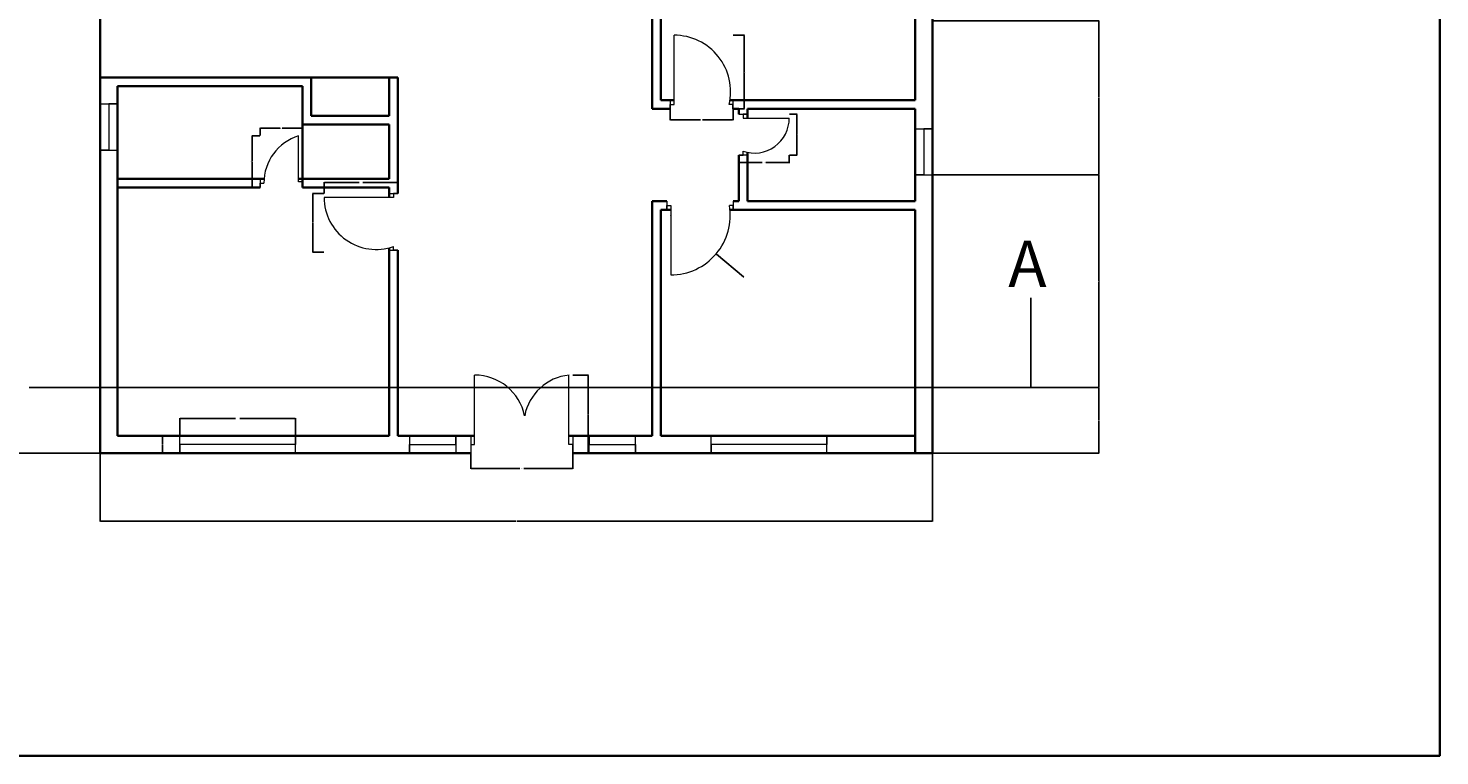
# Model space of a CAD drawing. Units: inches. Extents: x 2250 to 3547, y 1387 to 2604.
# Tile 4 of 11: x 2814 to 3547, y 1387 to 1765. Entities that reach past the tile are written whole.
import ezdxf

# ---------------------------------------------------------------- set-up
doc = ezdxf.new("R2010")
doc.units = ezdxf.units.IN
for name, color, linetype, lineweight in [('A-ANNO-DIMS', 2, 'Continuous', 18), ('A-ANNO-SYMB', 2, 'Continuous', 25), ('A-ANNO-TTLB', 7, 'Continuous', 35), ('A-DOOR', 3, 'Continuous', 18), ('A-GLAZ', 4, 'Continuous', 18), ('A-WALL', 7, 'Continuous', 35)]:
    doc.layers.add(name, color=color, linetype=linetype, lineweight=lineweight)
doc.styles.get("Standard").update_dxf_attribs({"font": 'arial.ttf'})
doc.dimstyles.get("Standard").update_dxf_attribs({"dimtxt": 0.18, "dimasz": 0.18, "dimexe": 0.18, "dimexo": 0.0625, "dimgap": 0.09, "dimtad": 0, "dimtih": 1, "dimtoh": 1, "dimdec": 4, "dimzin": 0, "dimdsep": 46, "dimtxsty": 'Standard', "dimcen": 0.09, "dimadec": 0, "dimazin": 0, "dimtfac": 1, "dimtdec": 4, "dimtofl": 0, "dimtmove": 0, "dimatfit": 3, "dimfxl": 1, "dimtolj": 1, "dimtzin": 0, "dimarcsym": 0})

# ---------------------------------------------------------------- blocks, each defined once
blk = doc.blocks.new('WIN-24')
for p, q in [((0, 24), (9, 24)), ((9, 24), (4.5, 24)), ((4.5, 24), (4.5, 0)), ((4.5, 0), (0, 0)), ((0, 0), (9, 0))]:
    blk.add_line(p, q)
blk = doc.blocks.new('WIN-60')
for p, q in [((0, 9), (0, 0)), ((60, 4.5), (60, 9)), ((60, 9), (60, 0)), ((0, 0), (0, 4.5)), ((0, 4.5), (60, 4.5))]:
    blk.add_line(p, q)
blk = doc.blocks.new('WIN-24-SPLIT')
for p, q in [((0, 9), (0, 0)), ((24, 4.5), (24, 9)), ((24, 9), (24, 0)), ((0, 0), (0, 4.5)), ((0, 4.5), (12, 4.5)), ((12, 4.5), (24, 4.5))]:
    blk.add_line(p, q)
blk = doc.blocks.new('DOOR-ENTRY-DOUBLE-SOUTH')
for p, q in [((2, 4.5), (2, 40.5)), ((51.02, 4.5), (51.02, 40.5)), ((0, 9), (0, 0)), ((53.02, 9), (53.02, 0)), ((0, 4.5), (2, 4.5)), ((53.02, 4.5), (51.02, 4.5)), ((53.02, 0), (53.02, 4.5))]:
    blk.add_line(p, q)
for centre, radius, start, end in [((2, 13.91), 26.59, 11.96772, 90), ((53.68, 14.51), 26.13, 95.82556, 169.16203)]:
    blk.add_arc(centre, radius, start, end)
blk = doc.blocks.new('DOOR-BED-SOUTHEAST')
for p, q in [((0, 38.25), (0, 33.75)), ((34.44, 38.25), (34.44, 33.75)), ((0, 33.75), (0, 36)), ((0, 36), (2, 36)), ((2, 36), (2, 0)), ((34.44, 36), (32.44, 36)), ((34.44, 33.75), (34.44, 36))]:
    blk.add_line(p, q)
blk.add_arc((2, 30.87), 30.87, 270, 9.55888)
blk = doc.blocks.new('DOOR-BED-WEST-S')
for p, q in [((33.75, 29.39), (38.25, 29.39)), ((38.25, 29.39), (36, 29.39)), ((36, 29.39), (36, 27.39)), ((36, 27.39), (0, 27.39)), ((36, 0), (36, 2)), ((33.75, 0), (38.25, 0)), ((38.25, 0), (36, 0))]:
    blk.add_line(p, q)
blk.add_arc((26.95, 27.39), 26.95, 180, 289.61215)
blk = doc.blocks.new('DOOR-BED-EAST-S')
for p, q in [((2, 2.25), (2, 38.25)), ((0, 4.5), (0, 0)), ((0, 0), (0, 2.25)), ((0, 2.25), (2, 2.25)), ((32.6, 2.25), (30.6, 2.25)), ((32.6, 4.5), (32.6, 0)), ((32.6, 0), (32.6, 2.25))]:
    blk.add_line(p, q)
blk.add_arc((2, 8.89), 29.36, 346.92103, 90)
blk = doc.blocks.new('DOOR-BATH-EAST-S')
for p, q in [((0, 21.23), (4.5, 21.23)), ((4.5, 21.23), (2.25, 21.23)), ((2.25, 21.23), (2.25, 19.23)), ((2.25, 19.23), (26.25, 19.23)), ((4.5, 0), (0, 0)), ((0, 0), (2.25, 0)), ((2.25, 0), (2.25, 2))]:
    blk.add_line(p, q)
blk.add_arc((8.07, 19.23), 18.18, 251.33598, 0)
blk = doc.blocks.new('DOOR-BATH-WEST-S')
for p, q in [((19.98, 2.81), (19.98, 26.81)), ((0, 4.5), (0, 0)), ((0, 0), (0, 2.25)), ((0, 2.25), (2, 2.25)), ((21.98, 2.81), (19.98, 2.81)), ((21.98, 0), (21.98, 2.81))]:
    blk.add_line(p, q)
blk.add_arc((27.76, 2.25), 25.76, 107.58549, 180)
blk = doc.blocks.new('*D28')
at = {"layer": 'A-ANNO-DIMS', "color": 0, "lineweight": -2, "transparency": 16777216}
for p, q in [((2893.03, 1552.99), (2893.03, 1562.1)), ((2893.21, 1561.92), (2921.91, 1561.92)), ((2952.85, 1561.92), (2924.15, 1561.92)), ((2953.03, 1552.99), (2953.03, 1562.1))]:
    blk.add_line(p, q, dxfattribs=at)
at = {"layer": 'A-ANNO-DIMS', "color": 0, "transparency": 16777216}
for points in [[(2893.21, 1561.95), (2893.21, 1561.89), (2893.03, 1561.92)], [(2952.85, 1561.95), (2952.85, 1561.89), (2953.03, 1561.92)]]:
    blk.add_solid(points, dxfattribs=at)
at = {"layer": 'Defpoints', "color": 0, "transparency": 16777216}
for p in [(2893.03, 1561.92), (2893.03, 1552.92), (2953.03, 1552.92)]:
    blk.add_point(p, dxfattribs=at)
at = {"layer": 'A-ANNO-DIMS', "color": 0, "transparency": 16777216, "insert": (2923.03, 1561.92), "char_height": 0.18, "attachment_point": 5}
blk.add_mtext('\\A1;WINDOW 60 TYP.', dxfattribs=at)
blk = doc.blocks.new('*D29')
at = {"layer": 'A-ANNO-DIMS', "color": 0, "lineweight": -2, "transparency": 16777216}
for p, q in [((2892.97, 1552.92), (2883.85, 1552.92)), ((2884.03, 1552.74), (2884.03, 1548.61)), ((2884.03, 1544.1), (2884.03, 1548.24)), ((2892.97, 1543.92), (2883.85, 1543.92))]:
    blk.add_line(p, q, dxfattribs=at)
at = {"layer": 'A-ANNO-DIMS', "color": 0, "transparency": 16777216}
for points in [[(2884, 1552.74), (2884.06, 1552.74), (2884.03, 1552.92)], [(2884, 1544.1), (2884.06, 1544.1), (2884.03, 1543.92)]]:
    blk.add_solid(points, dxfattribs=at)
at = {"layer": 'Defpoints', "color": 0, "transparency": 16777216}
for p in [(2893.03, 1552.92), (2884.03, 1543.92), (2893.03, 1543.92)]:
    blk.add_point(p, dxfattribs=at)
at = {"layer": 'A-ANNO-DIMS', "color": 0, "transparency": 16777216, "insert": (2884.03, 1548.42), "char_height": 0.18, "attachment_point": 5}
blk.add_mtext('\\A1;9 TYP.', dxfattribs=at)
blk = doc.blocks.new('*D42')
at = {"layer": 'A-ANNO-DIMS', "color": 0, "lineweight": -2, "transparency": 16777216}
for p, q in [((3043.99, 1543.86), (3043.99, 1535.79)), ((3097.02, 1543.86), (3097.02, 1535.79)), ((3044.17, 1535.97), (3069.52, 1535.97)), ((3096.84, 1535.97), (3071.49, 1535.97))]:
    blk.add_line(p, q, dxfattribs=at)
at = {"layer": 'A-ANNO-DIMS', "color": 0, "transparency": 16777216}
for points in [[(3044.17, 1536), (3044.17, 1535.94), (3043.99, 1535.97)], [(3096.84, 1536), (3096.84, 1535.94), (3097.02, 1535.97)]]:
    blk.add_solid(points, dxfattribs=at)
at = {"layer": 'Defpoints', "color": 0, "transparency": 16777216}
for p in [(3043.99, 1543.92), (3097.02, 1543.92), (3097.02, 1535.97)]:
    blk.add_point(p, dxfattribs=at)
at = {"layer": 'A-ANNO-DIMS', "color": 0, "transparency": 16777216, "insert": (3070.5, 1535.97), "char_height": 0.18, "attachment_point": 5}
blk.add_mtext('\\A1;ENTRY 53 TYP.', dxfattribs=at)
blk = doc.blocks.new('*D43')
at = {"layer": 'A-ANNO-DIMS', "color": 0, "lineweight": -2, "transparency": 16777216}
for p, q in [((3097.08, 1584.42), (3105.15, 1584.42)), ((3104.97, 1584.24), (3104.97, 1564.35)), ((3104.97, 1544.1), (3104.97, 1563.99)), ((3097.08, 1543.92), (3105.15, 1543.92))]:
    blk.add_line(p, q, dxfattribs=at)
at = {"layer": 'A-ANNO-DIMS', "color": 0, "transparency": 16777216}
for points in [[(3104.94, 1584.24), (3105, 1584.24), (3104.97, 1584.42)], [(3104.94, 1544.1), (3105, 1544.1), (3104.97, 1543.92)]]:
    blk.add_solid(points, dxfattribs=at)
at = {"layer": 'Defpoints', "color": 0, "transparency": 16777216}
for p in [(3097.02, 1584.42), (3104.97, 1584.42), (3097.02, 1543.92)]:
    blk.add_point(p, dxfattribs=at)
at = {"layer": 'A-ANNO-DIMS', "color": 0, "transparency": 16777216, "insert": (3104.97, 1564.17), "char_height": 0.18, "attachment_point": 5}
blk.add_mtext('\\A1;41 TYP.', dxfattribs=at)
blk = doc.blocks.new('*D50')
at = {"layer": 'A-ANNO-DIMS', "color": 0, "lineweight": -2, "transparency": 16777216}
for p, q in [((2967.88, 1678.73), (2967.88, 1684.59)), ((2968.06, 1684.41), (2986.07, 1684.41)), ((3005.95, 1684.41), (2987.94, 1684.41)), ((3006.13, 1678.73), (3006.13, 1684.59))]:
    blk.add_line(p, q, dxfattribs=at)
at = {"layer": 'A-ANNO-DIMS', "color": 0, "transparency": 16777216}
for points in [[(2968.06, 1684.44), (2968.06, 1684.38), (2967.88, 1684.41)], [(3005.95, 1684.44), (3005.95, 1684.38), (3006.13, 1684.41)]]:
    blk.add_solid(points, dxfattribs=at)
at = {"layer": 'Defpoints', "color": 0, "transparency": 16777216}
for p in [(2967.88, 1678.67), (3006.13, 1684.41), (3006.13, 1678.67)]:
    blk.add_point(p, dxfattribs=at)
at = {"layer": 'A-ANNO-DIMS', "color": 0, "transparency": 16777216, "insert": (2987, 1684.41), "char_height": 0.18, "attachment_point": 5}
blk.add_mtext('\\A1;DOOR 38 TYP.', dxfattribs=at)
blk = doc.blocks.new('*D51')
at = {"layer": 'A-ANNO-DIMS', "color": 0, "lineweight": -2, "transparency": 16777216}
for p, q in [((2967.82, 1678.67), (2961.96, 1678.67)), ((2962.14, 1678.49), (2962.14, 1663.69)), ((2962.14, 1648.52), (2962.14, 1663.32)), ((2967.82, 1648.34), (2961.96, 1648.34))]:
    blk.add_line(p, q, dxfattribs=at)
at = {"layer": 'A-ANNO-DIMS', "color": 0, "transparency": 16777216}
for points in [[(2962.11, 1678.49), (2962.17, 1678.49), (2962.14, 1678.67)], [(2962.11, 1648.52), (2962.17, 1648.52), (2962.14, 1648.34)]]:
    blk.add_solid(points, dxfattribs=at)
at = {"layer": 'Defpoints', "color": 0, "transparency": 16777216}
for p in [(2962.14, 1678.67), (2967.88, 1678.67), (2967.88, 1648.34)]:
    blk.add_point(p, dxfattribs=at)
at = {"layer": 'A-ANNO-DIMS', "color": 0, "transparency": 16777216, "insert": (2962.14, 1663.5), "char_height": 0.18, "attachment_point": 5}
blk.add_mtext('\\A1;30 TYP.', dxfattribs=at)
blk = doc.blocks.new('*D58')
at = {"layer": 'A-ANNO-DIMS', "color": 0, "lineweight": -2, "transparency": 16777216}
for p, q in [((3180.21, 1760.95), (3186.07, 1760.95)), ((3185.89, 1760.77), (3185.89, 1742)), ((3185.89, 1722.88), (3185.89, 1741.64)), ((3180.21, 1722.7), (3186.07, 1722.7))]:
    blk.add_line(p, q, dxfattribs=at)
at = {"layer": 'A-ANNO-DIMS', "color": 0, "transparency": 16777216}
for points in [[(3185.86, 1760.77), (3185.92, 1760.77), (3185.89, 1760.95)], [(3185.86, 1722.88), (3185.92, 1722.88), (3185.89, 1722.7)]]:
    blk.add_solid(points, dxfattribs=at)
at = {"layer": 'Defpoints', "color": 0, "transparency": 16777216}
for p in [(3180.15, 1760.95), (3185.89, 1760.95), (3180.15, 1722.7)]:
    blk.add_point(p, dxfattribs=at)
at = {"layer": 'A-ANNO-DIMS', "color": 0, "transparency": 16777216, "insert": (3185.89, 1741.82), "char_height": 0.18, "attachment_point": 5}
blk.add_mtext('\\A1;DOOR 38 TYP.', dxfattribs=at)
blk = doc.blocks.new('*D59')
at = {"layer": 'A-ANNO-DIMS', "color": 0, "lineweight": -2, "transparency": 16777216}
for p, q in [((3147.53, 1722.63), (3147.53, 1716.78)), ((3180.15, 1722.63), (3180.15, 1716.78)), ((3147.71, 1716.96), (3163.31, 1716.96)), ((3179.97, 1716.96), (3164.37, 1716.96))]:
    blk.add_line(p, q, dxfattribs=at)
at = {"layer": 'A-ANNO-DIMS', "color": 0, "transparency": 16777216}
for points in [[(3147.71, 1716.99), (3147.71, 1716.93), (3147.53, 1716.96)], [(3179.97, 1716.99), (3179.97, 1716.93), (3180.15, 1716.96)]]:
    blk.add_solid(points, dxfattribs=at)
at = {"layer": 'Defpoints', "color": 0, "transparency": 16777216}
for p in [(3147.53, 1722.7), (3180.15, 1722.7), (3180.15, 1716.96)]:
    blk.add_point(p, dxfattribs=at)
at = {"layer": 'A-ANNO-DIMS', "color": 0, "transparency": 16777216, "insert": (3163.84, 1716.96), "char_height": 0.18, "attachment_point": 5}
blk.add_mtext('\\A1;33 TYP.', dxfattribs=at)
blk = doc.blocks.new('*D62')
at = {"layer": 'A-ANNO-DIMS', "color": 0, "lineweight": -2, "transparency": 16777216}
for p, q in [((3183.13, 1698.63), (3183.13, 1694.58)), ((3183.31, 1694.76), (3195.32, 1694.76)), ((3209.2, 1694.76), (3197.19, 1694.76)), ((3209.38, 1698.63), (3209.38, 1694.58))]:
    blk.add_line(p, q, dxfattribs=at)
at = {"layer": 'A-ANNO-DIMS', "color": 0, "transparency": 16777216}
for points in [[(3183.31, 1694.79), (3183.31, 1694.73), (3183.13, 1694.76)], [(3209.2, 1694.79), (3209.2, 1694.73), (3209.38, 1694.76)]]:
    blk.add_solid(points, dxfattribs=at)
at = {"layer": 'Defpoints', "color": 0, "transparency": 16777216}
for p in [(3183.13, 1698.7), (3209.38, 1698.7), (3209.38, 1694.76)]:
    blk.add_point(p, dxfattribs=at)
at = {"layer": 'A-ANNO-DIMS', "color": 0, "transparency": 16777216, "insert": (3196.25, 1694.76), "char_height": 0.18, "attachment_point": 5}
blk.add_mtext('\\A1;DOOR 26 TYP.', dxfattribs=at)
blk = doc.blocks.new('*D63')
at = {"layer": 'A-ANNO-DIMS', "color": 0, "lineweight": -2, "transparency": 16777216}
for p, q in [((3209.44, 1719.92), (3213.5, 1719.92)), ((3213.32, 1719.74), (3213.32, 1709.49)), ((3213.32, 1698.88), (3213.32, 1709.13)), ((3209.44, 1698.7), (3213.5, 1698.7))]:
    blk.add_line(p, q, dxfattribs=at)
at = {"layer": 'A-ANNO-DIMS', "color": 0, "transparency": 16777216}
for points in [[(3213.29, 1719.74), (3213.35, 1719.74), (3213.32, 1719.92)], [(3213.29, 1698.88), (3213.35, 1698.88), (3213.32, 1698.7)]]:
    blk.add_solid(points, dxfattribs=at)
at = {"layer": 'Defpoints', "color": 0, "transparency": 16777216}
for p in [(3209.38, 1719.92), (3213.32, 1719.92), (3209.38, 1698.7)]:
    blk.add_point(p, dxfattribs=at)
at = {"layer": 'A-ANNO-DIMS', "color": 0, "transparency": 16777216, "insert": (3213.32, 1709.31), "char_height": 0.18, "attachment_point": 5}
blk.add_mtext('\\A1;21 TYP.', dxfattribs=at)
blk = doc.blocks.new('*D66')
at = {"layer": 'A-ANNO-DIMS', "color": 0, "lineweight": -2, "transparency": 16777216}
for p, q in [((2934.59, 1708.73), (2930.45, 1708.73)), ((2930.63, 1708.55), (2930.63, 1695.51)), ((2930.63, 1682.1), (2930.63, 1695.15)), ((2934.59, 1681.92), (2930.45, 1681.92))]:
    blk.add_line(p, q, dxfattribs=at)
at = {"layer": 'A-ANNO-DIMS', "color": 0, "transparency": 16777216}
for points in [[(2930.6, 1708.55), (2930.66, 1708.55), (2930.63, 1708.73)], [(2930.6, 1682.1), (2930.66, 1682.1), (2930.63, 1681.92)]]:
    blk.add_solid(points, dxfattribs=at)
at = {"layer": 'Defpoints', "color": 0, "transparency": 16777216}
for p in [(2930.63, 1708.73), (2934.65, 1708.73), (2934.65, 1681.92)]:
    blk.add_point(p, dxfattribs=at)
at = {"layer": 'A-ANNO-DIMS', "color": 0, "transparency": 16777216, "insert": (2930.63, 1695.33), "char_height": 0.18, "attachment_point": 5}
blk.add_mtext('\\A1;DOOR 27 TYP.', dxfattribs=at)
blk = doc.blocks.new('*D67')
at = {"layer": 'A-ANNO-DIMS', "color": 0, "lineweight": -2, "transparency": 16777216}
for p, q in [((2934.65, 1708.8), (2934.65, 1712.93)), ((2934.83, 1712.75), (2945.11, 1712.75)), ((2956.45, 1712.75), (2946.17, 1712.75)), ((2956.63, 1708.8), (2956.63, 1712.93))]:
    blk.add_line(p, q, dxfattribs=at)
at = {"layer": 'A-ANNO-DIMS', "color": 0, "transparency": 16777216}
for points in [[(2934.83, 1712.78), (2934.83, 1712.72), (2934.65, 1712.75)], [(2956.45, 1712.78), (2956.45, 1712.72), (2956.63, 1712.75)]]:
    blk.add_solid(points, dxfattribs=at)
at = {"layer": 'Defpoints', "color": 0, "transparency": 16777216}
for p in [(2934.65, 1708.73), (2956.63, 1712.75), (2956.63, 1708.73)]:
    blk.add_point(p, dxfattribs=at)
at = {"layer": 'A-ANNO-DIMS', "color": 0, "transparency": 16777216, "insert": (2945.64, 1712.75), "char_height": 0.18, "attachment_point": 5}
blk.add_mtext('\\A1;22 TYP.', dxfattribs=at)
blk = doc.blocks.new('*D84')
at = {"layer": 'A-ANNO-DIMS', "color": 0, "lineweight": -2, "transparency": 16777216}
for p, q in [((2851.63, 1543.86), (2851.63, 1508.39)), ((3283.63, 1543.86), (3283.63, 1508.39)), ((2851.81, 1508.57), (3067.34, 1508.57)), ((3283.45, 1508.57), (3067.92, 1508.57))]:
    blk.add_line(p, q, dxfattribs=at)
at = {"layer": 'A-ANNO-DIMS', "color": 0, "transparency": 16777216}
for points in [[(2851.81, 1508.6), (2851.81, 1508.54), (2851.63, 1508.57)], [(3283.45, 1508.6), (3283.45, 1508.54), (3283.63, 1508.57)]]:
    blk.add_solid(points, dxfattribs=at)
at = {"layer": 'Defpoints', "color": 0, "transparency": 16777216}
for p in [(2851.63, 1543.92), (3283.63, 1543.92), (3283.63, 1508.57)]:
    blk.add_point(p, dxfattribs=at)
at = {"layer": 'A-ANNO-DIMS', "color": 0, "transparency": 16777216, "insert": (3067.63, 1508.57), "char_height": 0.18, "attachment_point": 5}
blk.add_mtext('\\A1;432', dxfattribs=at)
blk = doc.blocks.new('*D85')
at = {"layer": 'A-ANNO-DIMS', "color": 0, "lineweight": -2, "transparency": 16777216}
for p, q in [((3001.57, 2245.18), (2779.34, 2245.18)), ((2779.52, 2245), (2779.52, 1894.73)), ((2779.52, 1544.1), (2779.52, 1894.37)), ((2851.57, 1543.92), (2779.34, 1543.92))]:
    blk.add_line(p, q, dxfattribs=at)
at = {"layer": 'A-ANNO-DIMS', "color": 0, "transparency": 16777216}
for points in [[(2779.49, 2245), (2779.55, 2245), (2779.52, 2245.18)], [(2779.49, 1544.1), (2779.55, 1544.1), (2779.52, 1543.92)]]:
    blk.add_solid(points, dxfattribs=at)
at = {"layer": 'Defpoints', "color": 0, "transparency": 16777216}
for p in [(2779.52, 2245.18), (3001.63, 2245.18), (2851.63, 1543.92)]:
    blk.add_point(p, dxfattribs=at)
at = {"layer": 'A-ANNO-DIMS', "color": 0, "transparency": 16777216, "insert": (2779.52, 1894.55), "char_height": 0.18, "attachment_point": 5}
blk.add_mtext('\\A1;701.3', dxfattribs=at)
blk = doc.blocks.new('*D86')
at = {"layer": 'A-ANNO-DIMS', "color": 0, "lineweight": -2, "transparency": 16777216}
for p, q in [((3334.76, 1577.98), (3370.22, 1577.98)), ((3370.04, 1577.8), (3370.04, 1561.13)), ((3370.04, 1544.1), (3370.04, 1560.77)), ((3283.69, 1543.92), (3370.22, 1543.92))]:
    blk.add_line(p, q, dxfattribs=at)
at = {"layer": 'A-ANNO-DIMS', "color": 0, "transparency": 16777216}
for points in [[(3370.01, 1577.8), (3370.07, 1577.8), (3370.04, 1577.98)], [(3370.01, 1544.1), (3370.07, 1544.1), (3370.04, 1543.92)]]:
    blk.add_solid(points, dxfattribs=at)
at = {"layer": 'Defpoints', "color": 0, "transparency": 16777216}
for p in [(3334.69, 1577.98), (3283.63, 1543.92), (3370.04, 1543.92)]:
    blk.add_point(p, dxfattribs=at)
at = {"layer": 'A-ANNO-DIMS', "color": 0, "transparency": 16777216, "insert": (3370.04, 1560.95), "char_height": 0.18, "attachment_point": 5}
blk.add_mtext('\\A1;34.05', dxfattribs=at)
blk = doc.blocks.new('*D87')
at = {"layer": 'A-ANNO-DIMS', "color": 0, "lineweight": -2, "transparency": 16777216}
for p, q in [((3283.69, 1688.39), (3370.22, 1688.39)), ((3370.04, 1688.21), (3370.04, 1633.37)), ((3370.04, 1578.16), (3370.04, 1633)), ((3334.76, 1577.98), (3370.22, 1577.98))]:
    blk.add_line(p, q, dxfattribs=at)
at = {"layer": 'A-ANNO-DIMS', "color": 0, "transparency": 16777216}
for points in [[(3370.01, 1688.21), (3370.07, 1688.21), (3370.04, 1688.39)], [(3370.01, 1578.16), (3370.07, 1578.16), (3370.04, 1577.98)]]:
    blk.add_solid(points, dxfattribs=at)
at = {"layer": 'Defpoints', "color": 0, "transparency": 16777216}
for p in [(3283.63, 1688.39), (3370.04, 1688.39), (3334.69, 1577.98)]:
    blk.add_point(p, dxfattribs=at)
at = {"layer": 'A-ANNO-DIMS', "color": 0, "transparency": 16777216, "insert": (3370.04, 1633.18), "char_height": 0.18, "attachment_point": 5}
blk.add_mtext('\\A1;110.42', dxfattribs=at)
blk = doc.blocks.new('*D88')
at = {"layer": 'A-ANNO-DIMS', "color": 0, "lineweight": -2, "transparency": 16777216}
for p, q in [((3283.69, 1768.42), (3370.22, 1768.42)), ((3370.04, 1768.24), (3370.04, 1728.59)), ((3370.04, 1688.57), (3370.04, 1728.23)), ((3283.69, 1688.39), (3370.22, 1688.39))]:
    blk.add_line(p, q, dxfattribs=at)
at = {"layer": 'A-ANNO-DIMS', "color": 0, "transparency": 16777216}
for points in [[(3370.01, 1768.24), (3370.07, 1768.24), (3370.04, 1768.42)], [(3370.01, 1688.57), (3370.07, 1688.57), (3370.04, 1688.39)]]:
    blk.add_solid(points, dxfattribs=at)
at = {"layer": 'Defpoints', "color": 0, "transparency": 16777216}
for p in [(3283.63, 1768.42), (3370.04, 1768.42), (3283.63, 1688.39)]:
    blk.add_point(p, dxfattribs=at)
at = {"layer": 'A-ANNO-DIMS', "color": 0, "transparency": 16777216, "insert": (3370.04, 1728.41), "char_height": 0.18, "attachment_point": 5}
blk.add_mtext('\\A1;80.03', dxfattribs=at)
blk = doc.blocks.new('*D116')
at = {"layer": 'A-ANNO-DIMS', "color": 0, "lineweight": -2, "transparency": 16777216}
for p, q in [((3147.72, 1667.32), (3147.9, 1667.32)), ((3147.81, 1667.23), (3147.81, 1667.41)), ((3185.52, 1635.42), (3171.52, 1647.27)), ((3185.7, 1635.42), (3185.52, 1635.42))]:
    blk.add_line(p, q, dxfattribs=at)
at = {"layer": 'A-ANNO-DIMS', "color": 0, "transparency": 16777216}
blk.add_solid([(3171.54, 1647.29), (3171.5, 1647.24), (3171.38, 1647.38)], dxfattribs=at)
at = {"layer": 'Defpoints', "color": 0, "transparency": 16777216}
for p in [(3147.81, 1667.32), (3171.38, 1647.38)]:
    blk.add_point(p, dxfattribs=at)
at = {"layer": 'A-ANNO-DIMS', "color": 0, "transparency": 16777216, "insert": (3186.25, 1635.42), "char_height": 0.18, "attachment_point": 5}
blk.add_mtext('\\A1;R30.873', dxfattribs=at)

msp = doc.modelspace()

# ---------------------------------------------------------------- linework, layer by layer
at = {"layer": 'A-ANNO-SYMB'}
for p, q in [((3334.6941, 1577.9756), (3334.6941, 1624.6412)), ((2814.8665, 1577.9756), (3334.6941, 1577.9756))]:
    msp.add_line(p, q, dxfattribs=at)
at = {"layer": 'A-ANNO-TTLB'}
msp.add_lwpolyline([(2250.1093, 2604.1988), (3546.995, 2604.1988), (3546.995, 1386.7251), (2250.1093, 1386.7251)], close=True, dxfattribs=at)
at = {"layer": 'A-WALL'}
for p, q in [((3283.6288, 2232.5639), (3283.6288, 1543.9245)), ((3274.6288, 2037.5639), (3274.6288, 1727.1967)), ((3142.6288, 1856.1967), (3142.6288, 1727.1967)), ((2851.6288, 1827.4245), (2851.6288, 1543.9245)), ((2851.6288, 1827.4245), (2851.6288, 1543.9245)), ((3138.1288, 1818.5639), (3138.1288, 1722.6967)), ((2851.6288, 1738.9245), (3001.6288, 1738.9245)), ((2961.1288, 1719.0224), (2961.1288, 1738.9245)), ((3001.6288, 1738.9245), (3001.6288, 1719.0224)), ((3001.6288, 1738.9245), (3006.1288, 1738.9245)), ((3006.1288, 1738.9245), (3006.1288, 1678.669)), ((2860.6288, 1734.4245), (2860.6288, 1552.9245)), ((2860.6288, 1734.4245), (2956.6288, 1734.4245)), ((2860.6288, 1734.4245), (2860.6288, 1686.4245)), ((2860.6288, 1734.4245), (2956.6288, 1734.4245)), ((2956.6288, 1734.4245), (2956.6288, 1714.5224)), ((3142.6288, 1722.6967), (3138.1288, 1722.6967)), ((3149.53, 1727.1967), (3142.6288, 1727.1967)), ((3147.53, 1722.6967), (3142.6288, 1722.6967)), ((3274.6288, 1727.1967), (3178.5561, 1727.1967)), ((3183.1288, 1722.6967), (3180.1252, 1722.6967)), ((3183.1288, 1722.6967), (3183.1288, 1719.9221)), ((3274.6288, 1722.6967), (3187.6288, 1722.6967)), ((3187.6288, 1717.9221), (3187.6288, 1722.6967)), ((3274.6288, 1722.6967), (3274.6288, 1674.6967)), ((2956.6288, 1714.5224), (3001.6288, 1714.5224)), ((2956.6288, 1714.5224), (2956.6288, 1681.9245)), ((3001.6288, 1719.0224), (2961.1288, 1719.0224)), ((3001.6288, 1714.5224), (3001.6288, 1686.4245)), ((3187.6288, 1674.6967), (3187.6288, 1700.0941)), ((3183.1288, 1698.6967), (3183.1288, 1674.6967)), ((2860.6288, 1686.4245), (2936.7483, 1686.4245)), ((2954.6288, 1686.4245), (3001.6288, 1686.4245)), ((2860.6288, 1681.9245), (2934.6498, 1681.9245)), ((2956.6288, 1681.9245), (3001.6288, 1681.9245)), ((3001.6288, 1681.9245), (3001.6288, 1676.669)), ((3138.1288, 1674.6967), (3138.1288, 1552.9245)), ((3138.1288, 1674.6967), (3145.8063, 1674.6967)), ((3180.2508, 1674.6967), (3183.1288, 1674.6967)), ((3274.6288, 1674.6967), (3187.6288, 1674.6967)), ((3274.6288, 1674.6967), (3187.6288, 1674.6967)), ((3142.6288, 1670.1967), (3142.6288, 1552.9245)), ((3147.8063, 1670.1967), (3142.6288, 1670.1967)), ((3183.1288, 1670.1967), (3178.5452, 1670.1967)), ((3274.6288, 1670.1967), (3183.1288, 1670.1967)), ((3274.6288, 1670.1967), (3274.6288, 1543.9245)), ((3001.6288, 1650.587), (3001.6288, 1552.9245)), ((3006.1288, 1649.2795), (3006.1288, 1552.9245)), ((2860.6288, 1552.9245), (3001.6288, 1552.9245)), ((3006.1288, 1552.9245), (3045.9924, 1552.9245)), ((3095.0157, 1552.9245), (3138.1288, 1552.9245)), ((3142.6288, 1552.9245), (3274.6288, 1552.9245)), ((2851.6288, 1543.9245), (3043.9924, 1543.9245)), ((3097.0157, 1543.9245), (3283.6288, 1543.9245))]:
    msp.add_line(p, q, dxfattribs=at)

# ---------------------------------------------------------------- block references
at = {"layer": 'A-DOOR'}
for name, p in [('DOOR-BED-EAST-S', (3147.53, 1722.6967)), ('DOOR-BATH-EAST-S', (3183.1288, 1698.6967)), ('DOOR-BATH-WEST-S', (2934.6498, 1681.9245)), ('DOOR-BED-WEST-S', (2967.8788, 1649.2795)), ('DOOR-BED-SOUTHEAST', (3145.8063, 1636.4467)), ('DOOR-ENTRY-DOUBLE-SOUTH', (3043.9924, 1543.9245))]:
    msp.add_blockref(name, p, dxfattribs=at)
at = {"layer": 'A-GLAZ'}
for name, p in [('WIN-24', (2851.6288, 1701.3211)), ('WIN-24', (3274.6288, 1688.3924)), ('WIN-24-SPLIT', (3012.2604, 1543.9245))]:
    msp.add_blockref(name, p, dxfattribs=at)
for name, p, rotation in [('WIN-60', (2953.0299, 1552.9245), 180), ('WIN-24', (3129.4634, 1543.9245), 90.00000000000003), ('WIN-60', (3228.8349, 1552.9245), 180)]:
    msp.add_blockref(name, p, dxfattribs=dict(at, rotation=rotation))

# ---------------------------------------------------------------- texts
at = {"layer": 'A-ANNO-SYMB', "insert": (3323.0015, 1654.2084), "char_height": 24, "attachment_point": 1}
msp.add_mtext_dynamic_manual_height_columns('A', width=29.785639, gutter_width=12.5, heights=[0], dxfattribs=at)

# ---------------------------------------------------------------- dimensions: what is measured, and where the dimension line sits
at = {"layer": 'A-ANNO-DIMS'}
for base, p1, p2, override, picture, middle in [((2779.5165, 2245.1762), (2851.6288, 1543.9245), (3001.6288, 2245.1762), {"dimdec": 1, "dimlfac": 1, "dimrnd": 0, "dimzin": 0, "dimdsep": 46, "dimlunit": 2}, '*D85', (2779.5165, 1894.5504)), ((3370.0441, 1768.424), (3283.6288, 1688.3924), (3283.6288, 1768.424), {"dimdec": 2, "dimlfac": 1, "dimrnd": 0, "dimzin": 0, "dimdsep": 46, "dimlunit": 2}, '*D88', (3370.0441, 1728.4082)), ((3370.0441, 1688.3924), (3334.6941, 1577.9756), (3283.6288, 1688.3924), {"dimdec": 2, "dimlfac": 1, "dimrnd": 0, "dimzin": 0, "dimdsep": 46, "dimlunit": 2}, '*D87', (3370.0441, 1633.184)), ((3370.0441, 1543.9245), (3334.6941, 1577.9756), (3283.6288, 1543.9245), {"dimdec": 2, "dimlfac": 1, "dimrnd": 0, "dimzin": 0, "dimdsep": 46, "dimlunit": 2}, '*D86', (3370.0441, 1560.9501))]:
    dim = msp.add_linear_dim(base=base, p1=p1, p2=p2, angle=90, dimstyle='Standard', override=override, dxfattribs=at)
    dim.commit()
    dim.dimension.update_dxf_attribs({"geometry": picture, "text_midpoint": middle})
for base, p1, p2, angle, text, picture, middle in [((3185.8889, 1760.9467), (3180.1514, 1722.6967), (3180.1514, 1760.9467), 90, 'DOOR <> TYP.', '*D58', (3185.8889, 1741.8217)), ((3213.3163, 1719.9221), (3209.3788, 1698.6967), (3209.3788, 1719.9221), 90, '<> TYP.', '*D63', (3213.3163, 1709.3094)), ((2930.6285, 1708.7331), (2934.6498, 1681.9245), (2934.6498, 1708.7331), 90, 'DOOR <> TYP.', '*D66', (2930.6285, 1695.3288)), ((2962.1413, 1678.669), (2967.8788, 1648.3387), (2967.8788, 1678.669), 90, '<> TYP.', '*D51', (2962.1413, 1663.5039)), ((3104.969209212, 1584.4245446338), (3097.0157148552, 1543.9245446338), (3097.0157148552, 1584.4245446338), 90, '<> TYP.', '*D43', (3104.969209212, 1564.1745446338)), ((2893.0299, 1561.9245), (2953.0299, 1552.9245), (2893.0299, 1552.9245), 180, 'WINDOW <> TYP.', '*D28', (2923.0299, 1561.9245)), ((2884.0299, 1543.9245), (2893.0299, 1552.9245), (2893.0299, 1543.9245), 270, '<> TYP.', '*D29', (2884.0299, 1548.4245))]:
    dim = msp.add_linear_dim(base=base, p1=p1, p2=p2, angle=angle, text=text, dimstyle='Standard', override={"dimdec": 0, "dimlfac": 1, "dimrnd": 0, "dimzin": 0, "dimdsep": 46, "dimlunit": 2}, dxfattribs=at)
    dim.commit()
    dim.dimension.update_dxf_attribs({"geometry": picture, "text_midpoint": middle})
for base, p1, p2, text, picture, middle in [((3180.1514, 1716.9592), (3147.53, 1722.6967), (3180.1514, 1722.6967), '<> TYP.', '*D59', (3163.8407, 1716.9592)), ((2956.6288, 1712.7544), (2934.6498, 1708.7331), (2956.6288, 1708.7331), '<> TYP.', '*D67', (2945.6393, 1712.7544)), ((3209.3788, 1694.7592), (3183.1288, 1698.6967), (3209.3788, 1698.6967), 'DOOR <> TYP.', '*D62', (3196.2538, 1694.7592)), ((3006.1288, 1684.4065), (2967.8788, 1678.669), (3006.1288, 1678.669), 'DOOR <> TYP.', '*D50', (2987.0038, 1684.4065)), ((3097.0157, 1535.9711), (3043.9924, 1543.9245), (3097.0157, 1543.9245), 'ENTRY <> TYP.', '*D42', (3070.5041, 1535.9711))]:
    dim = msp.add_linear_dim(base=base, p1=p1, p2=p2, text=text, dimstyle='Standard', override={"dimdec": 0, "dimlfac": 1, "dimrnd": 0, "dimzin": 0, "dimdsep": 46, "dimlunit": 2}, dxfattribs=at)
    dim.commit()
    dim.dimension.update_dxf_attribs({"geometry": picture, "text_midpoint": middle})
dim = msp.add_radius_dim(center=(3147.8063, 1667.3198), mpoint=(3171.38, 1647.384), dimstyle='Standard', override={"dimdec": 3, "dimlfac": 1, "dimrnd": 0, "dimzin": 0, "dimdsep": 46, "dimlunit": 2}, dxfattribs=at)
dim.commit()
dim.dimension.update_dxf_attribs({"geometry": '*D116', "text_midpoint": (3186.2539, 1635.4226), "dimtype": 164})
dim = msp.add_linear_dim(base=(3283.6288, 1508.5745), p1=(2851.6288, 1543.9245), p2=(3283.6288, 1543.9245), dimstyle='Standard', override={"dimdec": 0, "dimlfac": 1, "dimrnd": 0, "dimzin": 0, "dimdsep": 46, "dimlunit": 2}, dxfattribs=at)
dim.commit()
dim.dimension.update_dxf_attribs({"geometry": '*D84', "text_midpoint": (3067.6288, 1508.5745)})

doc.saveas('drawing.dxf')
